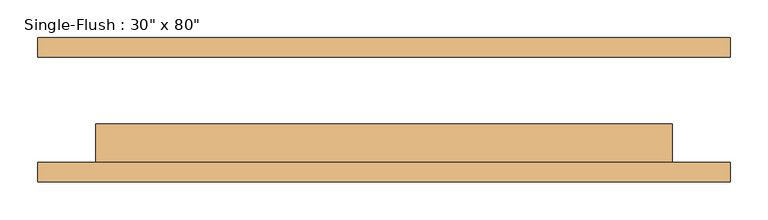
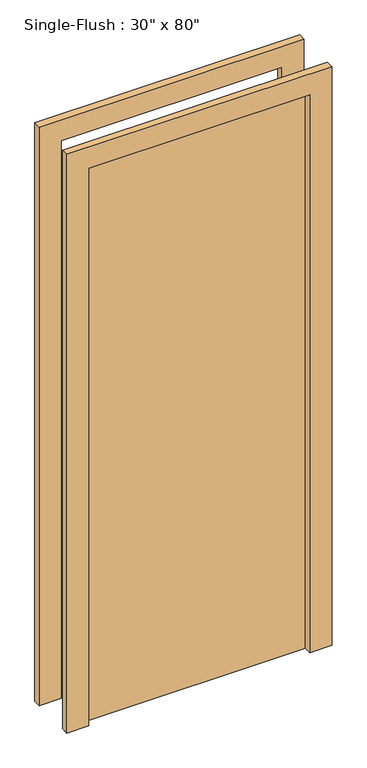
"""IFC4 building model written with IfcOpenShell, lengths in millimetres: door geometry."""

from ifc_helpers import new_model, si_unit, frame, origin, origin_with_axes, place, context, project, spatial, polyline, outline, extrude, source, transform, mapped, element, save


def door_c78455d5(model_context):
    return source(origin(), model_context, "Body", "SweptSolid", [
        extrude(outline(polyline([(2108.2, -457.2), (0.0, -457.2), (0.0, -381.0), (2032.0, -381.0), (2032.0, 381.0), (0.0, 381.0), (0.0, 457.2), (2108.2, 457.2), (2108.2, -457.2)])), frame((0.0, -95.25, 0.0), z_axis=(0.0, 1.0, 0.0), x_axis=(0.0, 0.0, 1.0)), (0.0, 0.0, 1.0), 25.4),
        extrude(outline(polyline([(2108.2, 457.2), (2108.2, -457.2), (0.0, -457.2), (0.0, -381.0), (2032.0, -381.0), (2032.0, 381.0), (0.0, 381.0), (0.0, 457.2), (2108.2, 457.2)])), frame((0.0, 69.85, 0.0), z_axis=(0.0, 1.0, 0.0), x_axis=(0.0, 0.0, 1.0)), (0.0, 0.0, 1.0), 25.4),
        extrude(outline(polyline([(381.0, -19.05), (381.0, -69.85), (-381.0, -69.85), (-381.0, -19.05), (381.0, -19.05)])), origin_with_axes(), (0.0, 0.0, 1.0), 2032.0),
    ])


if __name__ == "__main__":
    model = new_model("IFC4")
    model_context = context("Model", 3, world=origin())
    ifc_project = project(units=[si_unit("LENGTHUNIT", "METRE", prefix="MILLI")], contexts=[model_context])
    site = spatial("IfcSite", under=ifc_project)
    building = spatial("IfcBuilding", under=site)
    placement = place(None, origin())
    door_shape = door_c78455d5(model_context)
    element("IfcDoor", 1, ObjectType="Single-Flush : 30\" x 80\"", at=placement, inside=building, context=model_context, shape_type="MappedRepresentation", body=[
        mapped(door_shape, transform((0.0, 0.0, 0.0), x_axis=(1.0, 0.0, 0.0), y_axis=(0.0, 1.0, 0.0), z_axis=(0.0, 0.0, 1.0))),
    ])
    save(model, "model.ifc")

# Revit data of these elements
# Type "Single-Flush : 30\" x 80\""
#   Type Mark = "5"
#   Construction Type Id = "MDOOR"
#   Assembly Code = "C1020"
#   Analytic Construction = "Metal"
#   Thickness = 2"
#   Heat Transfer Coefficient (U) = 0.651978 BTU/(h·ft²·°F)
#   Height = 80"
#   Trim Projection Ext = 1"
#   Trim Projection Int = 1"
#   Trim Width = 3"
#   Width = 30"
#   Define Thermal Properties by = 1
#   Define Thermal Properties by = 1
#   Door Material = Door - Panel
#   Frame Material = Door - Frame
#   Visual Light Transmittance = 0
#   Solar Heat Gain Coefficient = 0
#   Function = (empty or 0)
#   Wall Closure = (empty or 0)
# Element 1 (IfcDoor, "Single-Flush : 30\" x 80\"")
#   Materials on its faces: "Door - Frame", "Door - Panel"
# Materials
#   "Door - Panel": class "Wood", colour RGB 210 159 95, transparency 0, Cost = 0
#   "Door - Frame": colour RGB 118 70 51, transparency 0, Cost = 0
